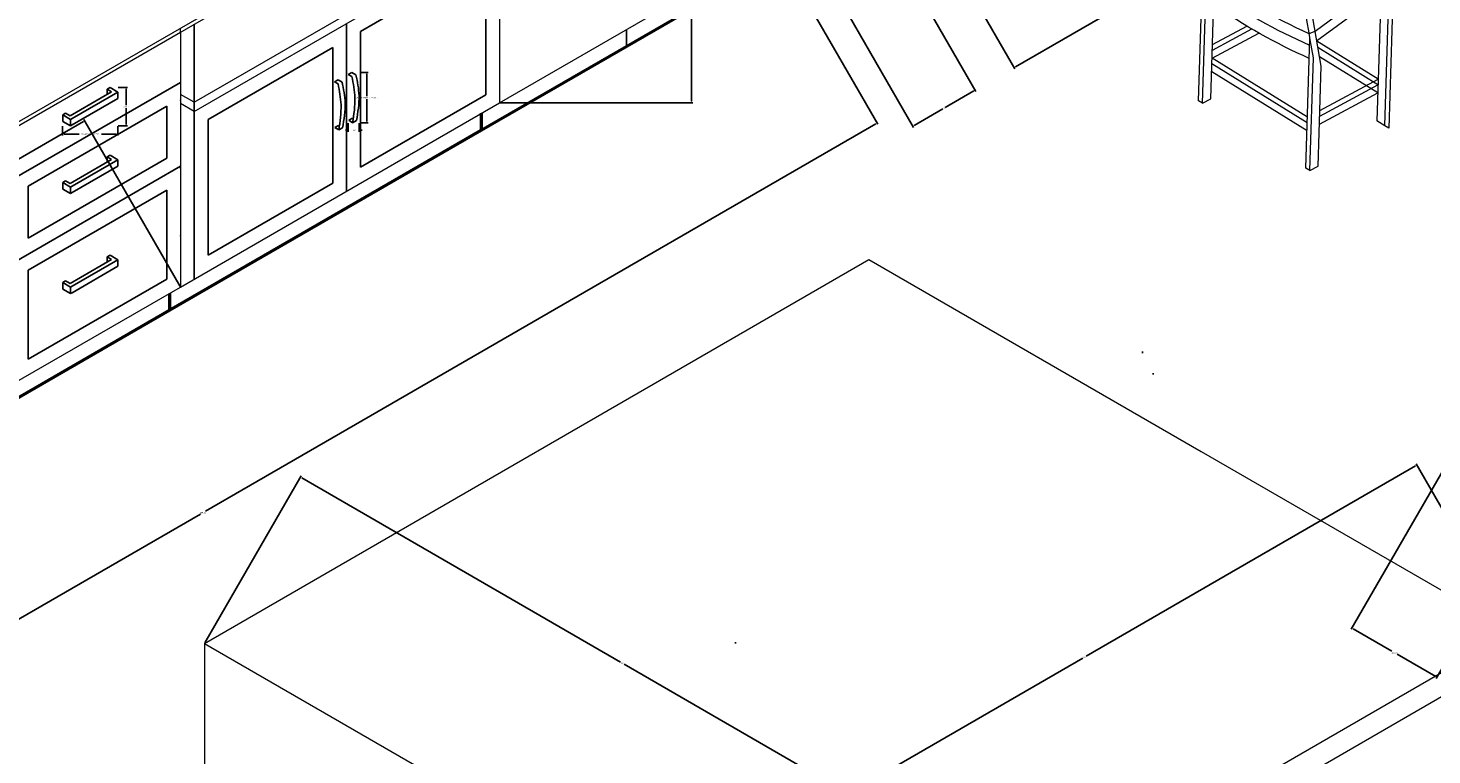
# Model space of a CAD drawing. Units: inches. Extents: x 4150 to 4636, y 2169 to 2592.
# Tile 5 of 8: x 4286 to 4462, y 2337 to 2428. Entities that reach past the tile are written whole.
import ezdxf

# ---------------------------------------------------------------- set-up
doc = ezdxf.new("R2010")
doc.units = ezdxf.units.IN
for name, color, linetype, lineweight in [('A-ANNO-DIMS', 2, 'Continuous', 18), ('A-CONS', 9, 'Continuous', 13), ('A-EQPM', 6, 'Continuous', 25), ('A-FLOR-CASE', 3, 'Continuous', 25), ('A-FLOR-FIXT', 8, 'Continuous', 18), ('A-FURN', 8, 'Continuous', 18), ('A-WALL', 7, 'Continuous', 50)]:
    doc.layers.add(name, color=color, linetype=linetype, lineweight=lineweight)
doc.styles.get("Standard").update_dxf_attribs({"font": 'arial.ttf'})
doc.dimstyles.get("Standard").update_dxf_attribs({"dimtxt": 0.18, "dimasz": 0.18, "dimexe": 0.18, "dimexo": 0.0625, "dimgap": 0.09, "dimtad": 0, "dimtih": 1, "dimtoh": 1, "dimdec": 4, "dimzin": 0, "dimdsep": 46, "dimtxsty": 'Standard', "dimcen": 0.09, "dimadec": 0, "dimazin": 0, "dimtfac": 1, "dimtdec": 4, "dimtofl": 0, "dimtmove": 0, "dimatfit": 3, "dimfxl": 1, "dimtolj": 1, "dimtzin": 0, "dimarcsym": 0})

# ---------------------------------------------------------------- blocks, each defined once
blk = doc.blocks.new('DRAG')
for p, q in [((4293.82, 2417.84), (4299.02, 2420.84)), ((4299.79, 2420.81), (4294.07, 2417.5)), ((4298.45, 2421.16), (4298.82, 2421.37)), ((4299.02, 2420.84), (4298.45, 2421.16)), ((4298.45, 2421.16), (4298.45, 2420.51)), ((4298.82, 2421.37), (4299.79, 2420.81)), ((4299.79, 2420.81), (4299.79, 2420)), ((4299.79, 2420), (4294.07, 2416.69)), ((4292.9, 2417.95), (4293.26, 2418.16)), ((4293.87, 2417.39), (4292.9, 2417.95)), ((4292.9, 2417.95), (4292.9, 2417.14)), ((4293.26, 2418.16), (4293.82, 2417.84)), ((4294.07, 2417.5), (4293.87, 2417.39)), ((4293.87, 2417.39), (4293.87, 2416.58)), ((4293.87, 2416.58), (4292.9, 2417.14)), ((4294.07, 2416.69), (4293.87, 2416.58))]:
    blk.add_line(p, q)
blk = doc.blocks.new('CHAIR')
for p, q in [((4460.61, 2323.17), (4462.07, 2322.64)), ((4459.26, 2268.31), (4459.26, 2302.96)), ((4458.4, 2267.81), (4458.4, 2298.32)), ((4419.13, 2296.33), (4418.72, 2294.28)), ((4435.02, 2283.82), (4419.13, 2296.33)), ((4434.61, 2281.77), (4418.72, 2294.28)), ((4418.72, 2294.28), (4418.72, 2263.74)), ((4419.58, 2264.24), (4419.58, 2293.6)), ((4421.31, 2292.24), (4421.31, 2265.24)), ((4456.67, 2268.81), (4456.67, 2290.03)), ((4436.24, 2283.27), (4435.02, 2283.82)), ((4456.67, 2277.45), (4446.94, 2283.07)), ((4456.67, 2279.13), (4448.46, 2283.88)), ((4456.67, 2280.34), (4449.53, 2284.46)), ((4421.31, 2274.06), (4434.6, 2281.73)), ((4421.31, 2272.85), (4434.31, 2280.36)), ((4436.06, 2254.73), (4436.06, 2282.33)), ((4421.31, 2271.17), (4433.9, 2278.43)), ((4435.2, 2254.23), (4435.2, 2278.19)), ((4436.06, 2265.55), (4456.67, 2277.45)), ((4433.46, 2267.05), (4421.31, 2274.06)), ((4433.46, 2255.23), (4433.46, 2276.44)), ((4436.06, 2264.34), (4456.67, 2276.24)), ((4436.06, 2262.66), (4456.67, 2274.56)), ((4433.46, 2265.84), (4421.31, 2272.85)), ((4433.46, 2264.15), (4421.31, 2271.17)), ((4458.4, 2267.81), (4456.67, 2268.81)), ((4458.4, 2267.81), (4459.26, 2268.31)), ((4419.58, 2264.24), (4421.31, 2265.24)), ((4418.72, 2263.74), (4419.58, 2264.24)), ((4435.2, 2254.23), (4433.46, 2255.23)), ((4435.2, 2254.23), (4436.06, 2254.73))]:
    blk.add_line(p, q)
for centre, radius, start, end in [((4387.22, 2413.69), 116.53, 296.3285, 309.0347), ((4384.96, 2418.26), 122.84, 296.6652, 308.8825), ((4169.51, 2354.34), 294.27, 347.3763, 353.8153), ((4146.35, 2340.95), 294.27, 347.3385, 353.8153), ((4147.53, 2340.19), 294.27, 347.8382, 353.8153), ((4388.03, 2401.62), 127.8, 292.164, 302.9931), ((4388.03, 2399.21), 127.8, 292.0735, 302.6755), ((4387.7, 2396.31), 127.8, 292.2346, 302.6625)]:
    blk.add_arc(centre, radius, start, end)
blk.add_open_spline([(4419.13, 2296.33), (4419.73, 2299.09), (4421.22, 2306.03), (4435.02, 2305.47), (4437.67, 2317.36), (4445.4, 2317.24), (4446.24, 2314.8), (4446.7, 2313.47)], degree=3, knots=[0, 0, 0, 0, 7.695976, 19.302291, 31.993754, 35.157842, 38.967805, 38.967805, 38.967805, 38.967805])
blk = doc.blocks.new('CAB-HANDLE')
for p, q in [((0, 6.03), (0.46, 6.29)), ((0.45, 5.77), (0, 6.03)), ((0.46, 6.29), (0.96, 6)), ((0.07, 0.31), (0.52, 0.57)), ((0.54, 0), (0.07, 0.31)), ((0.52, 0.57), (0.62, 0.52)), ((1.03, 0.28), (0.54, 0))]:
    blk.add_line(p, q)
for points, knots in [([(0.45, 5.77), (0.62, 4.9), (1, 2.98), (0.7, 1.05), (0.54, 0)], [0, 0, 0, 0, 2.653773, 5.810661, 5.810661, 5.810661, 5.810661]), ([(0.96, 6), (1.14, 5.13), (1.52, 3.23), (1.2, 1.31), (1.03, 0.28)], [0, 0, 0, 0, 2.653773, 5.763421, 5.763421, 5.763421, 5.763421])]:
    blk.add_open_spline(points, degree=3, knots=knots)
blk = doc.blocks.new('*D20')
at = {"layer": 'A-ANNO-DIMS', "color": 0, "lineweight": -2, "transparency": 16777216}
for p, q in [((4290.35, 2415.48), (4290.35, 2414.33)), ((4297.25, 2415.48), (4297.25, 2414.33)), ((4290.53, 2414.51), (4292.41, 2414.51)), ((4297.07, 2414.51), (4295.2, 2414.51))]:
    blk.add_line(p, q, dxfattribs=at)
at = {"layer": 'A-ANNO-DIMS', "color": 0, "transparency": 16777216}
for points in [[(4290.53, 2414.54), (4290.53, 2414.48), (4290.35, 2414.51)], [(4297.07, 2414.54), (4297.07, 2414.48), (4297.25, 2414.51)]]:
    blk.add_solid(points, dxfattribs=at)
at = {"layer": 'Defpoints', "color": 0, "transparency": 16777216}
for p in [(4290.35, 2415.54), (4297.25, 2415.54), (4297.25, 2414.51)]:
    blk.add_point(p, dxfattribs=at)
at = {"layer": 'A-ANNO-DIMS', "color": 0, "transparency": 16777216, "insert": (4293.8, 2414.51), "char_height": 0.18, "attachment_point": 5}
blk.add_mtext('\\A1;DRAWER PULL 7 TYP.', dxfattribs=at)
blk = doc.blocks.new('*D21')
at = {"layer": 'A-ANNO-DIMS', "color": 0, "lineweight": -2, "transparency": 16777216}
for p, q in [((4297.31, 2420.33), (4298.47, 2420.33)), ((4298.29, 2420.15), (4298.29, 2418.12)), ((4298.29, 2415.72), (4298.29, 2417.75)), ((4297.31, 2415.54), (4298.47, 2415.54))]:
    blk.add_line(p, q, dxfattribs=at)
at = {"layer": 'A-ANNO-DIMS', "color": 0, "transparency": 16777216}
for points in [[(4298.26, 2420.15), (4298.32, 2420.15), (4298.29, 2420.33)], [(4298.26, 2415.72), (4298.32, 2415.72), (4298.29, 2415.54)]]:
    blk.add_solid(points, dxfattribs=at)
at = {"layer": 'Defpoints', "color": 0, "transparency": 16777216}
for p in [(4297.25, 2420.33), (4298.29, 2420.33), (4297.25, 2415.54)]:
    blk.add_point(p, dxfattribs=at)
at = {"layer": 'A-ANNO-DIMS', "color": 0, "transparency": 16777216, "insert": (4298.29, 2417.94), "char_height": 0.18, "attachment_point": 5}
blk.add_mtext('\\A1;5 TYP.', dxfattribs=at)
blk = doc.blocks.new('*D22')
at = {"layer": 'A-ANNO-DIMS', "color": 0, "lineweight": -2, "transparency": 16777216}
for p, q in [((4327.53, 2422.21), (4328.59, 2422.21)), ((4328.41, 2422.03), (4328.41, 2419.25)), ((4328.41, 2416.1), (4328.41, 2418.88)), ((4327.53, 2415.92), (4328.59, 2415.92))]:
    blk.add_line(p, q, dxfattribs=at)
at = {"layer": 'A-ANNO-DIMS', "color": 0, "transparency": 16777216}
for points in [[(4328.38, 2422.03), (4328.44, 2422.03), (4328.41, 2422.21)], [(4328.38, 2416.1), (4328.44, 2416.1), (4328.41, 2415.92)]]:
    blk.add_solid(points, dxfattribs=at)
at = {"layer": 'Defpoints', "color": 0, "transparency": 16777216}
for p in [(4327.46, 2422.21), (4328.41, 2422.21), (4327.46, 2415.92)]:
    blk.add_point(p, dxfattribs=at)
at = {"layer": 'A-ANNO-DIMS', "color": 0, "transparency": 16777216, "insert": (4328.41, 2419.07), "char_height": 0.18, "attachment_point": 5}
blk.add_mtext('\\A1;CABINET HANDLE 6 TYP.', dxfattribs=at)
blk = doc.blocks.new('*D23')
at = {"layer": 'A-ANNO-DIMS', "color": 0, "lineweight": -2, "transparency": 16777216}
for p, q in [((4326.09, 2415.86), (4326.09, 2414.8)), ((4327.46, 2415.86), (4327.46, 2414.8)), ((4325.91, 2414.98), (4325.73, 2414.98)), ((4327.64, 2414.98), (4327.82, 2414.98))]:
    blk.add_line(p, q, dxfattribs=at)
at = {"layer": 'A-ANNO-DIMS', "color": 0, "transparency": 16777216}
for points in [[(4325.91, 2415.01), (4325.91, 2414.95), (4326.09, 2414.98)], [(4327.64, 2415.01), (4327.64, 2414.95), (4327.46, 2414.98)]]:
    blk.add_solid(points, dxfattribs=at)
at = {"layer": 'Defpoints', "color": 0, "transparency": 16777216}
for p in [(4326.09, 2415.92), (4327.46, 2415.92), (4327.46, 2414.98)]:
    blk.add_point(p, dxfattribs=at)
at = {"layer": 'A-ANNO-DIMS', "color": 0, "transparency": 16777216, "insert": (4326.78, 2414.98), "char_height": 0.18, "attachment_point": 5}
blk.add_mtext('\\A1;1 TYP.', dxfattribs=at)
blk = doc.blocks.new('*D36')
at = {"layer": 'A-ANNO-DIMS', "color": 0, "lineweight": -2, "transparency": 16777216}
for p, q in [((4174.28, 2460.03), (4174.28, 2592.15)), ((4174.46, 2591.97), (4402.51, 2591.97)), ((4631.36, 2591.97), (4403.31, 2591.97)), ((4631.54, 2412.03), (4631.54, 2592.15))]:
    blk.add_line(p, q, dxfattribs=at)
at = {"layer": 'A-ANNO-DIMS', "color": 0, "transparency": 16777216}
for points in [[(4174.46, 2592), (4174.46, 2591.94), (4174.28, 2591.97)], [(4631.36, 2592), (4631.36, 2591.94), (4631.54, 2591.97)]]:
    blk.add_solid(points, dxfattribs=at)
at = {"layer": 'Defpoints', "color": 0, "transparency": 16777216}
for p in [(4631.54, 2591.97), (4174.28, 2459.97), (4631.54, 2411.97)]:
    blk.add_point(p, dxfattribs=at)
at = {"layer": 'A-ANNO-DIMS', "color": 0, "transparency": 16777216, "insert": (4402.91, 2591.97), "char_height": 0.18, "attachment_point": 5}
blk.add_mtext('\\A1;457.3', dxfattribs=at)
blk = doc.blocks.new('*D37')
at = {"layer": 'A-ANNO-DIMS', "color": 0, "lineweight": -2, "transparency": 16777216}
for p, q in [((4361.28, 2567.97), (4150.1, 2567.97)), ((4150.28, 2567.79), (4150.28, 2379.06)), ((4150.28, 2189.96), (4150.28, 2378.69)), ((4434.34, 2189.78), (4150.1, 2189.78))]:
    blk.add_line(p, q, dxfattribs=at)
at = {"layer": 'A-ANNO-DIMS', "color": 0, "transparency": 16777216}
for points in [[(4150.25, 2567.79), (4150.31, 2567.79), (4150.28, 2567.97)], [(4150.25, 2189.96), (4150.31, 2189.96), (4150.28, 2189.78)]]:
    blk.add_solid(points, dxfattribs=at)
at = {"layer": 'Defpoints', "color": 0, "transparency": 16777216}
for p in [(4361.34, 2567.97), (4150.28, 2189.78), (4434.4, 2189.78)]:
    blk.add_point(p, dxfattribs=at)
at = {"layer": 'A-ANNO-DIMS', "color": 0, "transparency": 16777216, "insert": (4150.28, 2378.87), "char_height": 0.18, "attachment_point": 5}
blk.add_mtext('\\A1;378.2', dxfattribs=at)
blk = doc.blocks.new('*D38')
at = {"layer": 'A-ANNO-DIMS', "color": 0, "lineweight": -2, "transparency": 16777216}
for p, q in [((4174.25, 2348.68), (4162.2, 2327.79)), ((4162.45, 2327.85), (4292.04, 2253.15)), ((4422.26, 2178.08), (4292.67, 2252.79)), ((4434.37, 2198.73), (4422.33, 2177.84))]:
    blk.add_line(p, q, dxfattribs=at)
at = {"layer": 'A-ANNO-DIMS', "color": 0, "transparency": 16777216}
for points in [[(4162.46, 2327.88), (4162.43, 2327.83), (4162.29, 2327.94)], [(4422.27, 2178.11), (4422.24, 2178.05), (4422.42, 2177.99)]]:
    blk.add_solid(points, dxfattribs=at)
at = {"layer": 'Defpoints', "color": 0, "transparency": 16777216}
for p in [(4174.28, 2348.74), (4162.29, 2327.94), (4434.4, 2198.78)]:
    blk.add_point(p, dxfattribs=at)
at = {"layer": 'A-ANNO-DIMS', "color": 0, "transparency": 16777216, "insert": (4292.35, 2252.97), "char_height": 0.18, "attachment_point": 5}
blk.add_mtext('\\A1;300.25', dxfattribs=at)
blk = doc.blocks.new('*D43')
at = {"layer": 'A-ANNO-DIMS', "color": 0, "lineweight": -2, "transparency": 16777216}
for p, q in [((4361.37, 2568.02), (4373.43, 2588.91)), ((4373.5, 2588.66), (4504.26, 2513.17)), ((4635.59, 2437.34), (4504.83, 2512.83)), ((4623.78, 2416.52), (4635.84, 2437.41))]:
    blk.add_line(p, q, dxfattribs=at)
at = {"layer": 'A-ANNO-DIMS', "color": 0, "transparency": 16777216}
for points in [[(4373.51, 2588.69), (4373.48, 2588.63), (4373.34, 2588.75)], [(4635.61, 2437.37), (4635.58, 2437.31), (4635.75, 2437.25)]]:
    blk.add_solid(points, dxfattribs=at)
at = {"layer": 'Defpoints', "color": 0, "transparency": 16777216}
for p in [(4361.34, 2567.97), (4635.75, 2437.25), (4623.75, 2416.47)]:
    blk.add_point(p, dxfattribs=at)
at = {"layer": 'A-ANNO-DIMS', "color": 0, "transparency": 16777216, "insert": (4504.54, 2513), "char_height": 0.18, "attachment_point": 5}
blk.add_mtext('\\A1;303', dxfattribs=at)
blk = doc.blocks.new('*D49')
at = {"layer": 'A-ANNO-DIMS', "color": 0, "lineweight": -2, "transparency": 16777216}
for p, q in [((4392.55, 2440.74), (4404.61, 2419.85)), ((4384.76, 2436.24), (4396.81, 2415.35)), ((4404.36, 2419.92), (4400.77, 2417.84)), ((4396.88, 2415.6), (4400.47, 2417.67))]:
    blk.add_line(p, q, dxfattribs=at)
at = {"layer": 'A-ANNO-DIMS', "color": 0, "transparency": 16777216}
for points in [[(4404.35, 2419.94), (4404.38, 2419.89), (4404.52, 2420.01)], [(4396.87, 2415.62), (4396.9, 2415.57), (4396.72, 2415.51)]]:
    blk.add_solid(points, dxfattribs=at)
at = {"layer": 'Defpoints', "color": 0, "transparency": 16777216}
for p in [(4392.52, 2440.79), (4384.72, 2436.29), (4396.72, 2415.51)]:
    blk.add_point(p, dxfattribs=at)
at = {"layer": 'A-ANNO-DIMS', "color": 0, "transparency": 16777216, "insert": (4400.62, 2417.76), "char_height": 0.18, "attachment_point": 5}
blk.add_mtext('\\A1;9', dxfattribs=at)
blk = doc.blocks.new('*D51')
at = {"layer": 'A-ANNO-DIMS', "color": 0, "lineweight": -2, "transparency": 16777216}
for p, q in [((4426.8, 2460.49), (4438.85, 2439.61)), ((4397.44, 2443.55), (4409.5, 2422.66)), ((4438.61, 2439.67), (4424.4, 2431.47)), ((4409.57, 2422.91), (4423.77, 2431.11))]:
    blk.add_line(p, q, dxfattribs=at)
at = {"layer": 'A-ANNO-DIMS', "color": 0, "transparency": 16777216}
for points in [[(4438.59, 2439.7), (4438.62, 2439.65), (4438.76, 2439.76)], [(4409.55, 2422.93), (4409.58, 2422.88), (4409.41, 2422.82)]]:
    blk.add_solid(points, dxfattribs=at)
at = {"layer": 'Defpoints', "color": 0, "transparency": 16777216}
for p in [(4426.76, 2460.55), (4397.41, 2443.6), (4409.41, 2422.82)]:
    blk.add_point(p, dxfattribs=at)
at = {"layer": 'A-ANNO-DIMS', "color": 0, "transparency": 16777216, "insert": (4424.09, 2431.29), "char_height": 0.18, "attachment_point": 5}
blk.add_mtext('\\A1;33.89', dxfattribs=at)
blk = doc.blocks.new('*D55')
at = {"layer": 'A-ANNO-DIMS', "color": 0, "lineweight": -2, "transparency": 16777216}
for p, q in [((4380.31, 2436.61), (4392.37, 2415.73)), ((4392.12, 2415.79), (4308.21, 2367.35)), ((4223.67, 2318.54), (4307.58, 2366.99)), ((4211.55, 2339.18), (4223.61, 2318.3))]:
    blk.add_line(p, q, dxfattribs=at)
at = {"layer": 'A-ANNO-DIMS', "color": 0, "transparency": 16777216}
for points in [[(4392.11, 2415.82), (4392.14, 2415.77), (4392.28, 2415.88)], [(4223.66, 2318.57), (4223.69, 2318.52), (4223.52, 2318.45)]]:
    blk.add_solid(points, dxfattribs=at)
at = {"layer": 'Defpoints', "color": 0, "transparency": 16777216}
for p in [(4380.28, 2436.67), (4211.52, 2339.24), (4223.52, 2318.45)]:
    blk.add_point(p, dxfattribs=at)
at = {"layer": 'A-ANNO-DIMS', "color": 0, "transparency": 16777216, "insert": (4307.9, 2367.17), "char_height": 0.18, "attachment_point": 5}
blk.add_mtext('\\A1;194.86', dxfattribs=at)
blk = doc.blocks.new('*D61')
at = {"layer": 'A-ANNO-DIMS', "color": 0, "lineweight": -2, "transparency": 16777216}
for p, q in [((4345.08, 2450.81), (4369.2, 2450.81)), ((4369.02, 2450.63), (4369.02, 2434.8)), ((4369.02, 2418.61), (4369.02, 2434.44)), ((4345.08, 2418.43), (4369.2, 2418.43))]:
    blk.add_line(p, q, dxfattribs=at)
at = {"layer": 'A-ANNO-DIMS', "color": 0, "transparency": 16777216}
for points in [[(4368.99, 2450.63), (4369.05, 2450.63), (4369.02, 2450.81)], [(4368.99, 2418.61), (4369.05, 2418.61), (4369.02, 2418.43)]]:
    blk.add_solid(points, dxfattribs=at)
at = {"layer": 'Defpoints', "color": 0, "transparency": 16777216}
for p in [(4345.02, 2450.81), (4345.02, 2418.43), (4369.02, 2418.43)]:
    blk.add_point(p, dxfattribs=at)
at = {"layer": 'A-ANNO-DIMS', "color": 0, "transparency": 16777216, "insert": (4369.02, 2434.62), "char_height": 0.18, "attachment_point": 5}
blk.add_mtext('\\A1;32.387', dxfattribs=at)
blk = doc.blocks.new('*D62')
at = {"layer": 'A-ANNO-DIMS', "color": 0, "lineweight": -2, "transparency": 16777216}
for p, q in [((4463.66, 2373.46), (4451.6, 2352.57)), ((4474.29, 2367.32), (4462.23, 2346.43)), ((4451.85, 2352.64), (4456.69, 2349.84)), ((4462.17, 2346.68), (4457.32, 2349.48))]:
    blk.add_line(p, q, dxfattribs=at)
at = {"layer": 'A-ANNO-DIMS', "color": 0, "transparency": 16777216}
for points in [[(4451.86, 2352.66), (4451.83, 2352.61), (4451.69, 2352.73)], [(4462.18, 2346.7), (4462.15, 2346.65), (4462.32, 2346.59)]]:
    blk.add_solid(points, dxfattribs=at)
at = {"layer": 'Defpoints', "color": 0, "transparency": 16777216}
for p in [(4463.69, 2373.51), (4474.32, 2367.37), (4451.69, 2352.73)]:
    blk.add_point(p, dxfattribs=at)
at = {"layer": 'A-ANNO-DIMS', "color": 0, "transparency": 16777216, "insert": (4457.01, 2349.66), "char_height": 0.18, "attachment_point": 5}
blk.add_mtext('\\A1;12.278', dxfattribs=at)
blk = doc.blocks.new('*D66')
at = {"layer": 'A-ANNO-DIMS', "color": 0, "lineweight": -2, "transparency": 16777216}
for p, q in [((4308.14, 2350.86), (4320.2, 2371.75)), ((4320.26, 2371.5), (4360.16, 2348.47)), ((4400.49, 2325.18), (4360.6, 2348.21)), ((4388.68, 2304.36), (4400.74, 2325.25))]:
    blk.add_line(p, q, dxfattribs=at)
at = {"layer": 'A-ANNO-DIMS', "color": 0, "transparency": 16777216}
for points in [[(4320.28, 2371.53), (4320.25, 2371.48), (4320.11, 2371.59)], [(4400.51, 2325.21), (4400.48, 2325.16), (4400.65, 2325.09)]]:
    blk.add_solid(points, dxfattribs=at)
at = {"layer": 'Defpoints', "color": 0, "transparency": 16777216}
for p in [(4308.11, 2350.81), (4400.65, 2325.09), (4388.65, 2304.31)]:
    blk.add_point(p, dxfattribs=at)
at = {"layer": 'A-ANNO-DIMS', "color": 0, "transparency": 16777216, "insert": (4360.38, 2348.34), "char_height": 0.18, "attachment_point": 5}
blk.add_mtext('\\A1;93', dxfattribs=at)
blk = doc.blocks.new('*D67')
at = {"layer": 'A-ANNO-DIMS', "color": 0, "lineweight": -2, "transparency": 16777216}
for p, q in [((4471.75, 2352.36), (4459.7, 2373.25)), ((4459.63, 2373), (4418.44, 2349.22)), ((4376.8, 2325.18), (4418, 2348.96)), ((4388.62, 2304.36), (4376.56, 2325.25))]:
    blk.add_line(p, q, dxfattribs=at)
at = {"layer": 'A-ANNO-DIMS', "color": 0, "transparency": 16777216}
for points in [[(4459.62, 2373.03), (4459.65, 2372.98), (4459.79, 2373.09)], [(4376.79, 2325.21), (4376.82, 2325.16), (4376.65, 2325.09)]]:
    blk.add_solid(points, dxfattribs=at)
at = {"layer": 'Defpoints', "color": 0, "transparency": 16777216}
for p in [(4459.79, 2373.09), (4471.79, 2352.31), (4388.65, 2304.31)]:
    blk.add_point(p, dxfattribs=at)
at = {"layer": 'A-ANNO-DIMS', "color": 0, "transparency": 16777216, "insert": (4418.22, 2349.09), "char_height": 0.18, "attachment_point": 5}
blk.add_mtext('\\A1;96', dxfattribs=at)
blk = doc.blocks.new('*D71')
at = {"layer": 'A-ANNO-DIMS', "color": 0, "lineweight": -2, "transparency": 16777216}
for p, q in [((4292.94, 2416.07), (4282.93, 2410.29)), ((4305.07, 2395.43), (4293.01, 2416.32)), ((4272.47, 2404.25), (4282.49, 2410.04)), ((4284.28, 2383.43), (4272.23, 2404.32))]:
    blk.add_line(p, q, dxfattribs=at)
at = {"layer": 'A-ANNO-DIMS', "color": 0, "transparency": 16777216}
for points in [[(4292.93, 2416.1), (4292.96, 2416.05), (4293.1, 2416.16)], [(4272.46, 2404.28), (4272.49, 2404.23), (4272.32, 2404.16)]]:
    blk.add_solid(points, dxfattribs=at)
at = {"layer": 'Defpoints', "color": 0, "transparency": 16777216}
for p in [(4293.1, 2416.16), (4305.1, 2395.38), (4284.32, 2383.38)]:
    blk.add_point(p, dxfattribs=at)
at = {"layer": 'A-ANNO-DIMS', "color": 0, "transparency": 16777216, "insert": (4282.71, 2410.16), "char_height": 0.18, "attachment_point": 5}
blk.add_mtext('\\A1;24', dxfattribs=at)
blk = doc.blocks.new('*D76')
at = {"layer": 'A-ANNO-DIMS', "color": 0, "lineweight": -2, "transparency": 16777216}
for p, q in [((4374.44, 2350.89), (4374.62, 2350.89)), ((4374.53, 2350.8), (4374.53, 2350.98)), ((4430.33, 2244.06), (4409.49, 2283.96)), ((4430.51, 2244.06), (4430.33, 2244.06))]:
    blk.add_line(p, q, dxfattribs=at)
at = {"layer": 'A-ANNO-DIMS', "color": 0, "transparency": 16777216}
blk.add_solid([(4409.52, 2283.97), (4409.46, 2283.95), (4409.41, 2284.12)], dxfattribs=at)
at = {"layer": 'Defpoints', "color": 0, "transparency": 16777216}
for p in [(4374.53, 2350.89), (4409.41, 2284.12)]:
    blk.add_point(p, dxfattribs=at)
at = {"layer": 'A-ANNO-DIMS', "color": 0, "transparency": 16777216, "insert": (4430.99, 2244.06), "char_height": 0.18, "attachment_point": 5}
blk.add_mtext('\\A1;R75.33', dxfattribs=at)
blk = doc.blocks.new('*D77')
at = {"layer": 'A-ANNO-DIMS', "color": 0, "lineweight": -2, "transparency": 16777216}
for p, q in [((4425.48, 2387.12), (4425.48, 2387.3)), ((4425.39, 2387.21), (4425.57, 2387.21)), ((4488.19, 2289.8), (4464.77, 2326.18)), ((4488.37, 2289.8), (4488.19, 2289.8))]:
    blk.add_line(p, q, dxfattribs=at)
at = {"layer": 'A-ANNO-DIMS', "color": 0, "transparency": 16777216}
blk.add_solid([(4464.8, 2326.19), (4464.75, 2326.16), (4464.68, 2326.33)], dxfattribs=at)
at = {"layer": 'Defpoints', "color": 0, "transparency": 16777216}
for p in [(4425.48, 2387.21), (4464.68, 2326.33)]:
    blk.add_point(p, dxfattribs=at)
at = {"layer": 'A-ANNO-DIMS', "color": 0, "transparency": 16777216, "insert": (4488.84, 2289.8), "char_height": 0.18, "attachment_point": 5}
blk.add_mtext('\\A1;R72.41', dxfattribs=at)
blk = doc.blocks.new('*D78')
at = {"layer": 'A-ANNO-DIMS', "color": 0, "lineweight": -2, "transparency": 16777216}
for p, q in [((4426.72, 2384.51), (4426.9, 2384.51)), ((4426.81, 2384.42), (4426.81, 2384.6)), ((4486.16, 2292.01), (4464, 2326.55)), ((4486.34, 2292.01), (4486.16, 2292.01))]:
    blk.add_line(p, q, dxfattribs=at)
at = {"layer": 'A-ANNO-DIMS', "color": 0, "transparency": 16777216}
blk.add_solid([(4464.03, 2326.56), (4463.98, 2326.53), (4463.9, 2326.7)], dxfattribs=at)
at = {"layer": 'Defpoints', "color": 0, "transparency": 16777216}
for p in [(4426.81, 2384.51), (4463.9, 2326.7)]:
    blk.add_point(p, dxfattribs=at)
at = {"layer": 'A-ANNO-DIMS', "color": 0, "transparency": 16777216, "insert": (4486.82, 2292.01), "char_height": 0.18, "attachment_point": 5}
blk.add_mtext('\\A1;R68.69', dxfattribs=at)

msp = doc.modelspace()

# ---------------------------------------------------------------- linework, layer by layer
at = {"layer": 'A-CONS'}
for p in [(4305.0998, 2418.7653), (4305.0998, 2410.2653), (4305.0998, 2401.7653)]:
    msp.add_point(p, dxfattribs=at)
at = {"layer": 'A-EQPM'}
msp.add_line((4360.9195, 2427.6061), (4360.9195, 2425.4928), dxfattribs=at)
at = {"layer": 'A-FLOR-CASE'}
for p, q in [((4327.6164, 2427.3519), (4343.2897, 2436.4009)), ((4343.2897, 2436.4009), (4343.2897, 2419.4275)), ((4306.805, 2428.2498), (4306.805, 2396.363)), ((4325.8844, 2428.3519), (4325.8844, 2407.3785)), ((4327.6164, 2427.3519), (4327.6164, 2410.3785)), ((4308.537, 2416.3364), (4324.1523, 2425.3519)), ((4324.1523, 2425.3519), (4324.1523, 2408.3785)), ((4305.0998, 2420.9804), (4284.3152, 2408.9804)), ((4327.6164, 2410.3785), (4343.2897, 2419.4275)), ((4303.3677, 2417.9804), (4286.0472, 2407.9804)), ((4303.3677, 2417.9804), (4303.3677, 2411.4804)), ((4308.537, 2416.3364), (4308.537, 2399.363)), ((4305.0998, 2410.4804), (4284.3152, 2398.4804)), ((4303.3677, 2411.4804), (4286.0472, 2401.4804)), ((4308.537, 2399.363), (4324.1523, 2408.3785)), ((4286.0472, 2407.9804), (4286.0472, 2401.4804)), ((4303.3677, 2407.4804), (4286.0472, 2397.4804)), ((4303.3677, 2407.4804), (4303.3677, 2396.3785)), ((4286.0472, 2397.4804), (4286.0472, 2386.3785)), ((4286.0472, 2386.3785), (4303.3677, 2396.3785))]:
    msp.add_line(p, q, dxfattribs=at)
at = {"layer": 'A-FLOR-FIXT'}
for p, q in [((4247.9421, 2394.2653), (4382.1261, 2471.7364)), ((4283.8821, 2415.5153), (4381.6931, 2471.9864)), ((4345.0218, 2450.3142), (4345.0218, 2418.4275)), ((4306.805, 2418.4909), (4345.0218, 2440.5554)), ((4306.805, 2417.3364), (4345.0218, 2439.4009)), ((4345.0218, 2418.4275), (4382.1261, 2439.8497)), ((4305.0998, 2427.2653), (4305.0998, 2427.7653)), ((4247.9421, 2394.2653), (4305.0998, 2427.2653)), ((4305.0998, 2427.2653), (4305.0998, 2395.3785)), ((4306.805, 2418.4909), (4305.0998, 2419.4754)), ((4305.0998, 2395.3785), (4345.0218, 2418.4275)), ((4306.805, 2417.3364), (4305.0998, 2418.3209)), ((4284.3152, 2383.3785), (4305.0998, 2395.3785))]:
    msp.add_line(p, q, dxfattribs=at)
at = {"layer": 'A-FURN'}
for p, q in [((4308.1074, 2350.8064), (4391.2458, 2398.8064)), ((4391.2458, 2398.8064), (4432.8151, 2374.8064)), ((4432.8151, 2374.8064), (4471.7862, 2352.3064)), ((4388.6478, 2304.3064), (4471.7862, 2352.3064)), ((4308.1074, 2350.8064), (4349.6766, 2326.8064)), ((4308.1074, 2350.8064), (4308.1074, 2302.8064)), ((4391.2458, 2302.8064), (4469.1881, 2347.8064))]:
    msp.add_line(p, q, dxfattribs=at)
at = {"layer": 'A-WALL'}
for p, q in [((4342.7355, 2414.9942), (4380.2767, 2436.6687)), ((4342.7355, 2417.1075), (4342.7355, 2414.9942)), ((4303.7162, 2392.4665), (4342.7355, 2414.9942)), ((4303.7162, 2394.5797), (4303.7162, 2392.4665)), ((4284.3152, 2381.2653), (4303.7162, 2392.4665))]:
    msp.add_line(p, q, dxfattribs=at)

# ---------------------------------------------------------------- block references
at = {"layer": 'A-FLOR-CASE'}
for name, p in [('CAB-HANDLE', (4324.355, 2415.0201)), ('CAB-HANDLE', (4326.093, 2415.921)), ('DRAG', (-2.5414, -1.041)), ('DRAG', (-2.5414, -9.5013)), ('DRAG', (-2.5414, -22.015))]:
    msp.add_blockref(name, p, dxfattribs=at)
at = {"layer": 'A-FURN', "xscale": -0.589443472789305, "yscale": 0.589443472789305, "zscale": 0.5894434727893052, "rotation": 358.2313469525009}
msp.add_blockref('CHAIR', (7018.4597, 1001.1473), dxfattribs=at)

# ---------------------------------------------------------------- dimensions: what is measured, and where the dimension line sits
at = {"layer": 'A-ANNO-DIMS'}
dim = msp.add_linear_dim(base=(4631.5414, 2591.9652), p1=(4174.28, 2459.9652), p2=(4631.5414, 2411.9652), dimstyle='Standard', override={"dimdec": 1, "dimlfac": 1, "dimrnd": 0, "dimzin": 0, "dimdsep": 46, "dimlunit": 2}, dxfattribs=at)
dim.commit()
dim.dimension.update_dxf_attribs({"geometry": '*D36', "text_midpoint": (4402.9107, 2591.9652)})
for base, p1, p2, angle, override, picture, middle in [((4635.7472, 2437.2498), (4361.3415, 2567.9652), (4623.7472, 2416.4652), 330, {"dimdec": 0, "dimlfac": 1, "dimrnd": 0, "dimzin": 0, "dimdsep": 46, "dimlunit": 2}, '*D43', (4504.5443, 2512.9998)), ((4150.28, 2189.7836), (4361.3415, 2567.9652), (4434.4021, 2189.7836), 90, {"dimdec": 1, "dimlfac": 1, "dimrnd": 0, "dimzin": 0, "dimdsep": 46, "dimlunit": 2}, '*D37', (4150.28, 2378.8744)), ((4409.4119, 2422.8168), (4426.7642, 2460.548), (4397.4119, 2443.6015), 210, {"dimdec": 2, "dimlfac": 1, "dimrnd": 0, "dimzin": 0, "dimdsep": 46, "dimlunit": 2}, '*D51', (4424.0881, 2431.2901)), ((4369.0218, 2418.4275), (4345.0218, 2450.8142), (4345.0218, 2418.4275), 270, {"dimdec": 3, "dimlfac": 1, "dimrnd": 0, "dimzin": 0, "dimdsep": 46, "dimlunit": 2}, '*D61', (4369.0218, 2434.6209)), ((4396.7242, 2415.508), (4392.5184, 2440.7926), (4384.7242, 2436.2926), 210, {"dimdec": 0, "dimlfac": 1, "dimrnd": 0, "dimzin": 0, "dimdsep": 46, "dimlunit": 2}, '*D49', (4400.6213, 2417.758)), ((4223.5191, 2318.4518), (4380.2767, 2436.6687), (4211.5191, 2339.2364), 210, {"dimdec": 2, "dimlfac": 1, "dimrnd": 0, "dimzin": 0, "dimdsep": 46, "dimlunit": 2}, '*D55', (4307.8979, 2367.1679)), ((4293.0998, 2416.1631), (4284.3152, 2383.3785), (4305.0998, 2395.3785), 30, {"dimdec": 0, "dimlfac": 1, "dimrnd": 0, "dimzin": 0, "dimdsep": 46, "dimlunit": 2}, '*D71', (4282.7075, 2410.1631)), ((4459.7862, 2373.091), (4388.6478, 2304.3064), (4471.7862, 2352.3064), 30, {"dimdec": 0, "dimlfac": 1, "dimrnd": 0, "dimzin": 0, "dimdsep": 46, "dimlunit": 2}, '*D67', (4418.217, 2349.091)), ((4451.6899, 2352.7265), (4474.3231, 2367.372), (4463.6899, 2373.5111), 150, {"dimdec": 3, "dimlfac": 1, "dimrnd": 0, "dimzin": 0, "dimdsep": 46, "dimlunit": 2}, '*D62', (4457.0065, 2349.657)), ((4400.6478, 2325.091), (4308.1074, 2350.8064), (4388.6478, 2304.3064), 330, {"dimdec": 0, "dimlfac": 1, "dimrnd": 0, "dimzin": 0, "dimdsep": 46, "dimlunit": 2}, '*D66', (4360.3776, 2348.341)), ((4162.2937, 2327.9439), (4434.4021, 2198.7836), (4174.28, 2348.7364), 150.037803, {"dimdec": 2, "dimlfac": 1, "dimrnd": 0, "dimzin": 0, "dimdsep": 46, "dimlunit": 2}, '*D38', (4292.3547, 2252.9675))]:
    dim = msp.add_linear_dim(base=base, p1=p1, p2=p2, angle=angle, dimstyle='Standard', override=override, dxfattribs=at)
    dim.commit()
    dim.dimension.update_dxf_attribs({"geometry": picture, "text_midpoint": middle})
for base, p1, p2, text, picture, middle in [((4328.4078, 2422.2137), (4327.4639, 2415.9209), (4327.4639, 2422.2137), 'CABINET HANDLE <> TYP.', '*D22', (4328.4078, 2419.0673)), ((4298.285, 2420.3306), (4297.2505, 2415.5399), (4297.2505, 2420.3306), '<> TYP.', '*D21', (4298.285, 2417.9353))]:
    dim = msp.add_linear_dim(base=base, p1=p1, p2=p2, angle=90, text=text, dimstyle='Standard', override={"dimdec": 0, "dimlfac": 1, "dimrnd": 0, "dimzin": 0, "dimdsep": 46, "dimlunit": 2}, dxfattribs=at)
    dim.commit()
    dim.dimension.update_dxf_attribs({"geometry": picture, "text_midpoint": middle})
for base, p1, p2, text, picture, middle in [((4297.2505, 2414.5054), (4290.3537, 2415.5399), (4297.2505, 2415.5399), 'DRAWER PULL <> TYP.', '*D20', (4293.8021, 2414.5054)), ((4327.4639, 2414.977), (4326.0932, 2415.9209), (4327.4639, 2415.9209), '<> TYP.', '*D23', (4326.7785, 2414.977))]:
    dim = msp.add_linear_dim(base=base, p1=p1, p2=p2, text=text, dimstyle='Standard', override={"dimdec": 0, "dimlfac": 1, "dimrnd": 0, "dimzin": 0, "dimdsep": 46, "dimlunit": 2}, dxfattribs=at)
    dim.commit()
    dim.dimension.update_dxf_attribs({"geometry": picture, "text_midpoint": middle})
for center, mpoint, picture, middle in [((4425.4794, 2387.2104), (4464.6759, 2326.3282), '*D77', (4488.8362, 2289.7989)), ((4426.8142, 2384.5135), (4463.904, 2326.699), '*D78', (4486.8179, 2292.0103)), ((4374.5318, 2350.8893), (4409.4062, 2284.1195), '*D76', (4430.9907, 2244.0577))]:
    dim = msp.add_radius_dim(center=center, mpoint=mpoint, dimstyle='Standard', override={"dimdec": 2, "dimlfac": 1, "dimrnd": 0, "dimzin": 0, "dimdsep": 46, "dimlunit": 2}, dxfattribs=at)
    dim.commit()
    dim.dimension.update_dxf_attribs({"geometry": picture, "text_midpoint": middle, "dimtype": 164})

doc.saveas('drawing.dxf')
